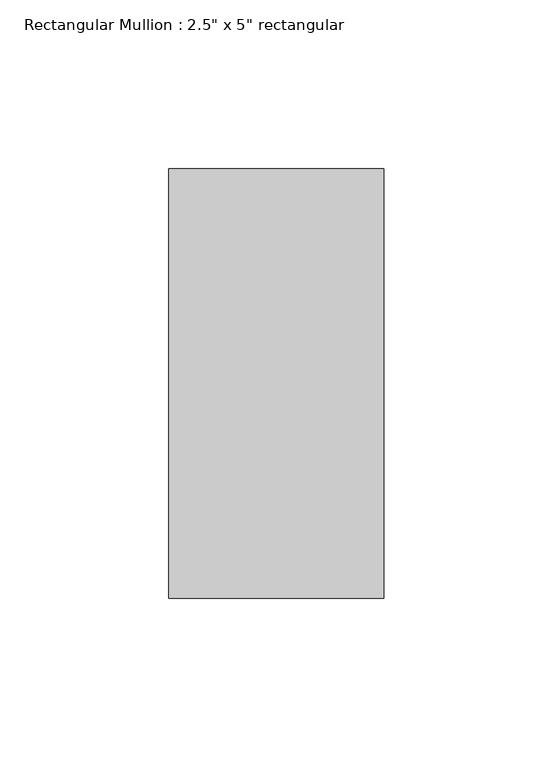
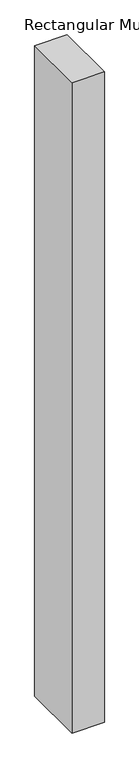
"""IFC4 building model written with IfcOpenShell, lengths in millimetres: member geometry."""

from ifc_helpers import new_model, si_unit, frame, origin, place, context, project, spatial, polyline, outline, extrude, source, transform, mapped, element, save


def member_5e346b9e(model_context):
    return source(origin(), model_context, "Body", "SweptSolid", [
        extrude(outline(polyline([(0.0, 63.5), (0.0, -63.5), (-63.5, -63.5), (-63.5, 63.5), (0.0, 63.5)])), frame((0.0, 0.0, -1351.2300456), z_axis=(0.0, 0.0, 1.0), x_axis=(1.0, 0.0, 0.0)), (0.0, 0.0, 1.0), 1351.2300456),
    ])


if __name__ == "__main__":
    model = new_model("IFC4")
    model_context = context("Model", 3, world=origin())
    ifc_project = project(units=[si_unit("LENGTHUNIT", "METRE", prefix="MILLI")], contexts=[model_context])
    site = spatial("IfcSite", under=ifc_project)
    building = spatial("IfcBuilding", under=site)
    placement = place(None, origin())
    member_shape = member_5e346b9e(model_context)
    element("IfcMember", 1, ObjectType="Rectangular Mullion : 2.5\" x 5\" rectangular", at=placement, inside=building, context=model_context, shape_type="MappedRepresentation", body=[
        mapped(member_shape, transform((0.0, 0.0, 0.0), x_axis=(1.0, 0.0, 0.0), y_axis=(0.0, 1.0, 0.0), z_axis=(0.0, 0.0, 1.0))),
    ])
    save(model, "model.ifc")

# Revit data of these elements
# Type "Rectangular Mullion : 2.5\" x 5\" rectangular"
#   built-in parameter 1007304 = 0.416667 (stored number, unit not read)
#   built-in parameter 1007301 = 0.104167 (stored number, unit not read)
#   built-in parameter 1007300 = 0.104167 (stored number, unit not read)
# Element 1 (IfcMember, "Rectangular Mullion : 2.5\" x 5\" rectangular")
#   Materials on its faces: "door colour"
# Materials
#   "door colour": class "Generic", colour RGB 120 120 120, transparency 0, Cost = 0
